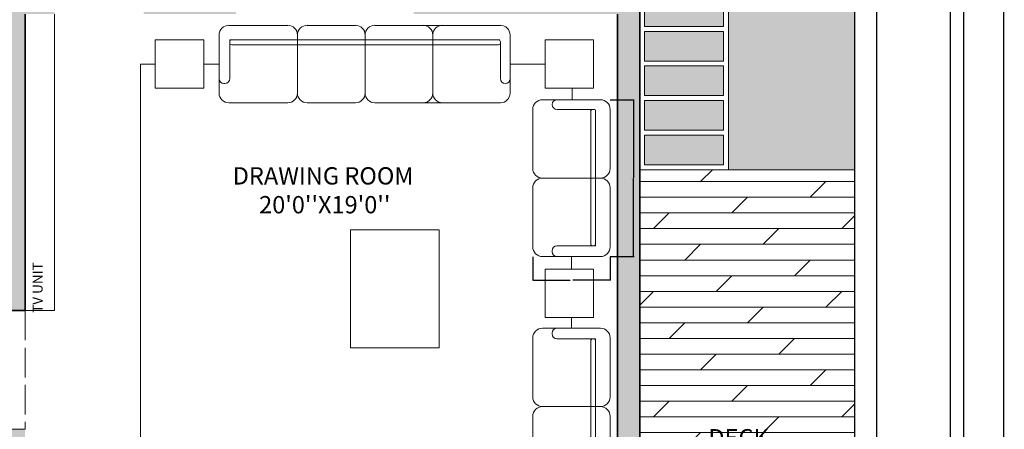
# Model space of a CAD drawing. Units: inches. Extents: x 84 to 1044, y -280 to 906.
# Tile 66 of 105: x 645 to 1044, y 160 to 326. Entities that reach past the tile are written whole.
import ezdxf

# ---------------------------------------------------------------- set-up
doc = ezdxf.new("R2010")
doc.units = ezdxf.units.IN
doc.linetypes.add('ACAD_ISO02W100', pattern=[15, 12, -3])
for name, color, linetype, lineweight in [('A-ANNO-DIMS', 2, 'Continuous', 18), ('A-ANNO-TEXT', 7, 'Continuous', 13), ('A-ANNO-TTLB', 7, 'Continuous', 25), ('A-AREA-IDEN', 7, 'Continuous', 13), ('A-FLOR-CASE', 8, 'Continuous', 18), ('A-FURN', 8, 'Continuous', 15), ('A-WALL-OVHD', 8, 'ACAD_ISO02W100', 13), ('C-PROP', 7, 'Continuous', 25), ('L-HRDS', 32, 'Continuous', 18), ('WALL', 250, 'Continuous', 35)]:
    doc.layers.add(name, color=color, linetype=linetype, lineweight=lineweight)
for name, color, linetype, lineweight, true_color in [('A-FLOR-PATT', 251, 'Continuous', 9, 0x705861), ('A-WALL-PATT', 251, 'Continuous', 9, 0x636466), ('L-HRDS-PATT', 23, 'Continuous', 9, 0xc2877b), ('L-PLNT-PATT', 9, 'Continuous', 9, 0xafd9aa)]:
    doc.layers.add(name, color=color, linetype=linetype, lineweight=lineweight, true_color=true_color)
doc.styles.add('1-100DIM', font='txt', dxfattribs={"height": 0.3})
doc.styles.get("Standard").update_dxf_attribs({"font": 'arial.ttf'})
doc.dimstyles.get("Standard").update_dxf_attribs({"dimtxt": 0.18, "dimasz": 0.18, "dimexe": 0.18, "dimexo": 0.0625, "dimgap": 0.09, "dimtad": 0, "dimtih": 1, "dimtoh": 1, "dimdec": 4, "dimzin": 0, "dimdsep": 46, "dimtxsty": 'Standard', "dimcen": 0.09, "dimadec": 0, "dimazin": 0, "dimtfac": 1, "dimtdec": 4, "dimtofl": 0, "dimtmove": 0, "dimatfit": 3, "dimfxl": 1, "dimtolj": 1, "dimtzin": 0, "dimarcsym": 0})

# ---------------------------------------------------------------- blocks, each defined once
blk = doc.blocks.new('SOFA-4-SEAT')
for p, q in [((3.92, 31.33), (27.81, 31.33)), ((27.81, 31.33), (27.81, 31.33)), ((35.65, 31.33), (55.23, 31.33)), ((55.23, 31.33), (55.23, 31.33)), ((63.07, 31.33), (113.96, 31.33)), ((113.96, 31.33), (113.96, 31.33)), ((0, 3.91), (0, 27.42)), ((4.31, 12.82), (4.31, 25.46)), ((4.31, 25.46), (11.69, 25.46)), ((4.31, 24.28), (4.31, 24.67)), ((5.09, 25.46), (11.69, 25.46)), ((11.69, 25.46), (113.76, 25.46)), ((11.69, 25.46), (113.18, 25.46)), ((31.73, 27.42), (31.73, 3.91)), ((31.73, 3.91), (31.73, 27.42)), ((59.15, 3.91), (59.15, 27.42)), ((59.15, 27.42), (59.15, 3.91)), ((86.57, 27.42), (86.57, 3.91)), ((113.96, 24.67), (113.96, 24.28)), ((113.96, 24.28), (113.96, 9.79)), ((117.88, 27.42), (117.88, 3.91)), ((13.66, 23.5), (5.09, 23.5)), ((113.18, 23.5), (13.66, 23.5)), ((4.31, 9.79), (4.31, 12.82)), ((1.96, 7.83), (2.35, 7.83)), ((115.92, 7.83), (115.92, 7.83)), ((27.81, 0), (3.92, 0)), ((27.81, 0), (27.81, 0)), ((55.23, 0), (35.65, 0)), ((55.23, 0), (55.23, 0)), ((113.96, 0), (63.07, 0)), ((113.96, 0), (113.96, 0))]:
    blk.add_line(p, q)
for centre, radius, start, end in [((3.92, 27.42), 3.92, 90, 180), ((27.81, 27.42), 3.92, 0, 90), ((35.65, 27.42), 3.92, 90, 180), ((55.23, 27.42), 3.92, 0, 90), ((63.07, 27.42), 3.92, 90, 180), ((82.65, 27.42), 3.92, 0, 90), ((90.48, 27.42), 3.92, 90, 180), ((113.96, 27.42), 3.92, 0, 90), ((5.09, 24.67), 0.783, 90, 180), ((5.09, 24.28), 0.783, 180, 270), ((113.18, 24.67), 0.783, 0, 90), ((113.18, 24.28), 0.783, 270, 0), ((1.96, 9.79), 1.96, 180, 270), ((2.35, 9.79), 1.96, 270, 0), ((115.92, 9.79), 1.96, 180, 270), ((115.92, 9.79), 1.96, 270, 0), ((3.92, 3.91), 3.92, 180, 270), ((27.81, 3.91), 3.92, 270, 0), ((35.65, 3.91), 3.92, 180, 270), ((55.23, 3.91), 3.92, 270, 0), ((63.07, 3.91), 3.92, 180, 270), ((82.65, 3.91), 3.92, 270, 0), ((90.48, 3.91), 3.92, 180, 270), ((113.96, 3.91), 3.92, 270, 0)]:
    blk.add_arc(centre, radius, start, end)
blk = doc.blocks.new('SOFA-2-SEAT')
for p, q in [((27.42, 63.46), (3.92, 63.46)), ((7.83, 61.5), (7.83, 61.5)), ((0, 59.54), (0, 59.54)), ((0, 59.54), (0, 35.65)), ((24.29, 59.54), (9.79, 59.54)), ((23.5, 58.76), (23.5, 13.66)), ((24.68, 59.54), (24.29, 59.54)), ((25.46, 11.69), (25.46, 59.35)), ((25.46, 11.69), (25.46, 58.76)), ((31.34, 59.54), (31.34, 59.54)), ((31.34, 35.65), (31.34, 59.54)), ((3.92, 31.73), (27.42, 31.73)), ((27.42, 31.73), (3.92, 31.73)), ((0, 27.81), (0, 27.81)), ((0, 27.81), (0, 3.92)), ((31.34, 27.81), (31.34, 27.81)), ((31.34, 3.92), (31.34, 27.81)), ((23.5, 13.66), (23.5, 5.09)), ((25.46, 5.09), (25.46, 11.69)), ((25.46, 4.31), (25.46, 11.69)), ((9.79, 4.31), (12.83, 4.31)), ((12.83, 4.31), (25.46, 4.31)), ((24.29, 4.31), (24.68, 4.31)), ((3.92, 0), (27.42, 0)), ((7.83, 1.96), (7.83, 2.35))]:
    blk.add_line(p, q)
for centre, radius, start, end in [((3.92, 59.54), 3.92, 90, 180), ((9.79, 61.5), 1.96, 90, 180), ((9.79, 61.5), 1.96, 180, 270), ((27.42, 59.54), 3.92, 360, 90), ((24.29, 58.76), 0.783, 90, 180), ((24.68, 58.76), 0.783, 360, 90), ((3.92, 35.65), 3.92, 180, 270), ((27.42, 35.65), 3.92, 270, 360), ((3.92, 27.81), 3.92, 90, 180), ((27.42, 27.81), 3.92, 360, 90), ((9.79, 2.35), 1.96, 90, 180), ((24.29, 5.09), 0.783, 180, 270), ((24.68, 5.09), 0.783, 270, 360), ((3.92, 3.92), 3.92, 180, 270), ((9.79, 1.96), 1.96, 180, 270), ((27.42, 3.92), 3.92, 270, 360)]:
    blk.add_arc(centre, radius, start, end)
blk = doc.blocks.new('TABLE-END-SQUARE')
for p, q in [((0, 0), (0, 19.59)), ((0, 19.59), (19.58, 19.59)), ((19.58, 19.59), (19.58, 0)), ((19.58, 0), (0, 0))]:
    blk.add_line(p, q)
blk = doc.blocks.new('PAVER-32X12')
blk.add_lwpolyline([(0, 12), (32, 12), (32, 0), (0, 0)], close=True)
blk = doc.blocks.new('*D54')
at = {"layer": 'A-ANNO-DIMS', "color": 0, "lineweight": -2, "transparency": 16777216}
for p, q in [((884.17, 293.48), (893.8, 293.48)), ((893.62, 293.3), (893.62, 261.93)), ((893.62, 230.2), (893.62, 261.57)), ((884.17, 230.02), (893.8, 230.02))]:
    blk.add_line(p, q, dxfattribs=at)
at = {"layer": 'A-ANNO-DIMS', "color": 0, "transparency": 16777216}
for points in [[(893.59, 293.3), (893.65, 293.3), (893.62, 293.48)], [(893.59, 230.2), (893.65, 230.2), (893.62, 230.02)]]:
    blk.add_solid(points, dxfattribs=at)
at = {"layer": 'Defpoints', "color": 0, "transparency": 16777216}
for p in [(884.11, 293.48), (893.62, 293.48), (884.11, 230.02)]:
    blk.add_point(p, dxfattribs=at)
at = {"layer": 'A-ANNO-DIMS', "color": 0, "transparency": 16777216, "insert": (893.62, 261.75), "char_height": 0.18, "attachment_point": 5}
blk.add_mtext('\\A1;LOVESEAT 63 TYP.', dxfattribs=at)
blk = doc.blocks.new('*D55')
at = {"layer": 'A-ANNO-DIMS', "color": 0, "lineweight": -2, "transparency": 16777216}
for p, q in [((852.77, 229.96), (852.77, 220.32)), ((884.11, 229.96), (884.11, 220.32)), ((852.95, 220.5), (867.91, 220.5)), ((883.93, 220.5), (868.97, 220.5))]:
    blk.add_line(p, q, dxfattribs=at)
at = {"layer": 'A-ANNO-DIMS', "color": 0, "transparency": 16777216}
for points in [[(852.95, 220.53), (852.95, 220.47), (852.77, 220.5)], [(883.93, 220.53), (883.93, 220.47), (884.11, 220.5)]]:
    blk.add_solid(points, dxfattribs=at)
at = {"layer": 'Defpoints', "color": 0, "transparency": 16777216}
for p in [(852.77, 230.02), (884.11, 230.02), (884.11, 220.5)]:
    blk.add_point(p, dxfattribs=at)
at = {"layer": 'A-ANNO-DIMS', "color": 0, "transparency": 16777216, "insert": (868.44, 220.5), "char_height": 0.18, "attachment_point": 5}
blk.add_mtext('\\A1;31 TYP.', dxfattribs=at)
blk = doc.blocks.new('*D63')
at = {"layer": 'A-ANNO-DIMS', "color": 0, "lineweight": -2, "transparency": 16777216}
for p, q in [((833.14, 709.12), (1043.77, 709.12)), ((1043.59, 708.94), (1043.59, 400.3)), ((1043.59, 91.3), (1043.59, 399.94)), ((896.14, 91.12), (1043.77, 91.12))]:
    blk.add_line(p, q, dxfattribs=at)
at = {"layer": 'A-ANNO-DIMS', "color": 0, "transparency": 16777216}
for points in [[(1043.56, 708.94), (1043.62, 708.94), (1043.59, 709.12)], [(1043.56, 91.3), (1043.62, 91.3), (1043.59, 91.12)]]:
    blk.add_solid(points, dxfattribs=at)
at = {"layer": 'Defpoints', "color": 0, "transparency": 16777216}
for p in [(833.07, 709.12), (1043.59, 709.12), (896.07, 91.12)]:
    blk.add_point(p, dxfattribs=at)
at = {"layer": 'A-ANNO-DIMS', "color": 0, "transparency": 16777216, "insert": (1043.59, 400.12), "char_height": 0.18, "attachment_point": 5}
blk.add_mtext('\\A1;618', dxfattribs=at)

msp = doc.modelspace()

# ---------------------------------------------------------------- hatches: boundary and pattern name
at = {"layer": 'A-FLOR-PATT', "transparency": 33554597}
h = msp.add_hatch(dxfattribs=at)
h.set_pattern_fill('DOLMIT', color=256)
h.paths.add_polyline_path([(983.074, 265.12), (896.074, 265.12), (896.074, 91.12), (887.074, 91.12), (887.074, 31.12), (983.074, 31.12)])
at = {"layer": 'A-WALL-PATT', "transparency": 33554597}
h = msp.add_hatch(color=256, dxfattribs=at)
h.dxf.hatch_style = 1
h.paths.add_polyline_path([(671.074, 100.12), (647.074, 100.12), (647.074, 160.12), (641.074, 160.12), (620.824, 160.12), (620.824, 151.12), (638.074, 151.12), (638.074, 91.12), (671.074, 91.12)])
h.paths.add_polyline_path([(791.074, 100.12), (743.074, 100.12), (743.074, 91.12), (791.074, 91.12)])
h.paths.add_polyline_path([(896.074, 346.12), (887.074, 346.12), (887.074, 334.12), (870.955, 334.12), (833.074, 334.12), (804.574, 334.12), (804.574, 328.12), (887.074, 328.12), (887.074, 100.12), (863.074, 100.12), (863.074, 91.12), (896.074, 91.12)])
h.paths.add_polyline_path([(507.574, 154.729), (507.574, 160.12), (464.074, 160.12), (464.074, 247.12), (641.074, 247.12), (641.074, 208.12), (647.074, 208.12), (647.074, 328.12), (659.074, 328.12), (659.074, 334.12), (617.074, 334.12), (617.074, 328.12), (641.074, 328.12), (641.074, 256.12), (545.074, 256.12), (545.074, 328.12), (569.074, 328.12), (569.074, 334.12), (518.074, 334.12), (518.074, 325.12), (536.074, 325.12), (536.074, 256.12), (464.074, 256.12), (464.074, 325.12), (482.074, 325.12), (482.074, 334.12), (455.074, 334.12), (455.074, 160.12), (413.127, 160.12), (413.127, 151.12), (455.074, 151.12), (455.074, 91.12), (464.074, 91.12), (464.074, 151.12), (507.574, 151.12)])
h.paths.add_polyline_path([(572.824, 160.12), (555.574, 160.12), (555.574, 151.12), (572.824, 151.12)], flags=17)
h.paths.add_polyline_path([(341.127, 160.12), (299.179, 160.12), (299.179, 211.12), (294.179, 211.12), (290.179, 211.12), (290.179, 151.12), (341.127, 151.12)])
h.paths.add_polyline_path([(299.179, 256.12), (212.179, 256.12), (212.179, 274.12), (203.179, 274.12), (203.179, 247.12), (299.179, 247.12)])
h.paths.add_polyline_path([(212.179, 514.12), (398.074, 514.12), (398.074, 519.12), (398.074, 520.12), (212.179, 520.12), (212.179, 574.12), (203.179, 574.12), (203.179, 310.12), (212.179, 310.12), (212.179, 328.12), (290.179, 328.12), (290.179, 292.12), (299.179, 292.12), (299.179, 328.12), (332.179, 328.12), (332.179, 334.12), (212.179, 334.12)])
h.paths.add_polyline_path([(287.127, 709.12), (203.179, 709.12), (203.179, 646.12), (212.179, 646.12), (212.179, 700.12), (287.127, 700.12)])
h.paths.add_polyline_path([(470.074, 709.12), (359.127, 709.12), (359.127, 700.12), (434.074, 700.12), (434.074, 574.12), (440.074, 574.12), (440.074, 622.12), (464.074, 622.12), (464.074, 628.12), (440.074, 628.12), (440.074, 700.12), (470.074, 700.12)])
h.paths.add_polyline_path([(572.074, 709.12), (506.074, 709.12), (506.074, 700.12), (536.074, 700.12), (536.074, 628.12), (494.074, 628.12), (494.074, 622.12), (536.074, 622.12), (536.074, 520.12), (440.074, 520.12), (440.074, 544.12), (434.074, 544.12), (434.074, 514.12), (644.074, 514.12), (644.074, 519.12), (644.074, 544.12), (638.074, 544.12), (638.074, 520.12), (542.074, 520.12), (542.074, 622.12), (584.074, 622.12), (584.074, 628.12), (542.074, 628.12), (542.074, 700.12), (572.074, 700.12)])
h.paths.add_polyline_path([(698.074, 709.12), (608.074, 709.12), (608.074, 700.12), (638.074, 700.12), (638.074, 628.12), (614.074, 628.12), (614.074, 622.12), (638.074, 622.12), (638.074, 574.12), (644.074, 574.12), (644.074, 700.12), (698.074, 700.12)])
h.paths.add_polyline_path([(833.074, 709.12), (770.074, 709.12), (770.074, 700.12), (824.074, 700.12), (824.074, 646.12), (833.074, 646.12)])
h.paths.add_polyline_path([(833.074, 574.12), (824.074, 574.12), (824.074, 520.12), (791.244, 520.12), (712.904, 520.12), (680.074, 520.12), (680.074, 514.12), (695.074, 514.12), (695.074, 491.62), (704.074, 491.62), (704.074, 511.12), (833.074, 511.12)])
h.paths.add_polyline_path([(704.074, 419.62), (695.074, 419.62), (695.074, 370.12), (704.074, 370.12)])
h.paths.add_polyline_path([(896.074, 400.12), (833.074, 400.12), (833.074, 364.12), (839.074, 364.12), (839.074, 394.12), (887.074, 394.12), (887.074, 382.12), (896.074, 382.12)])
h.paths.add_polyline_path([(732.574, 334.12), (695.074, 334.12), (695.074, 328.12), (732.574, 328.12)])
at = {"layer": 'L-HRDS-PATT', "transparency": 33554597}
h = msp.add_hatch(color=256, dxfattribs=at)
h.dxf.hatch_style = 1
h.paths.add_polyline_path([(930.074, 545.12), (898.074, 545.12), (898.074, 533.12), (930.074, 533.12)])
h.paths.add_polyline_path([(930.074, 531.12), (898.074, 531.12), (898.074, 519.12), (930.074, 519.12)])
h.paths.add_polyline_path([(930.074, 517.12), (898.074, 517.12), (898.074, 505.12), (930.074, 505.12)])
h.paths.add_polyline_path([(930.074, 503.12), (898.074, 503.12), (898.074, 491.12), (930.074, 491.12)])
h.paths.add_polyline_path([(930.074, 489.12), (898.074, 489.12), (898.074, 477.12), (930.074, 477.12)])
h.paths.add_polyline_path([(930.074, 475.12), (898.074, 475.12), (898.074, 463.12), (930.074, 463.12)])
h.paths.add_polyline_path([(930.074, 461.12), (898.074, 461.12), (898.074, 449.12), (930.074, 449.12)])
h.paths.add_polyline_path([(930.074, 447.12), (898.074, 447.12), (898.074, 435.12), (930.074, 435.12)])
h.paths.add_polyline_path([(930.074, 433.12), (898.074, 433.12), (898.074, 421.12), (930.074, 421.12)])
h.paths.add_polyline_path([(930.074, 419.12), (898.074, 419.12), (898.074, 407.12), (930.074, 407.12)])
h.paths.add_polyline_path([(930.074, 405.12), (898.074, 405.12), (898.074, 393.12), (930.074, 393.12)])
h.paths.add_polyline_path([(930.074, 391.12), (898.074, 391.12), (898.074, 379.12), (930.074, 379.12)])
h.paths.add_polyline_path([(930.074, 377.12), (898.074, 377.12), (898.074, 365.12), (930.074, 365.12)])
h.paths.add_polyline_path([(930.074, 363.12), (898.074, 363.12), (898.074, 351.12), (930.074, 351.12)])
h.paths.add_polyline_path([(930.074, 349.12), (898.074, 349.12), (898.074, 337.12), (930.074, 337.12)])
h.paths.add_polyline_path([(930.074, 335.12), (898.074, 335.12), (898.074, 323.12), (930.074, 323.12)])
h.paths.add_polyline_path([(930.074, 321.12), (898.074, 321.12), (898.074, 309.12), (930.074, 309.12)])
h.paths.add_polyline_path([(930.074, 307.12), (898.074, 307.12), (898.074, 295.12), (930.074, 295.12)])
h.paths.add_polyline_path([(930.074, 293.12), (898.074, 293.12), (898.074, 281.12), (930.074, 281.12)])
h.paths.add_polyline_path([(930.074, 279.12), (898.074, 279.12), (898.074, 267.12), (930.074, 267.12)])
at = {"layer": 'L-PLNT-PATT', "transparency": 33554597}
h = msp.add_hatch(color=256, dxfattribs=at)
h.dxf.hatch_style = 1
h.paths.add_polyline_path([(434.074, 769.12), (386.074, 769.12), (386.074, 709.12), (434.074, 709.12)])
h.paths.add_polyline_path([(896.074, 847.12), (434.074, 847.12), (434.074, 769.12), (434.074, 709.12), (470.074, 709.12), (506.074, 709.12), (572.074, 709.12), (608.074, 709.12), (698.074, 709.12), (770.074, 709.12), (833.074, 709.12), (896.074, 709.12)])
h.paths.add_polyline_path([(983.074, 847.12), (896.074, 847.12), (896.074, 709.12), (896.074, 547.12), (932.074, 547.12), (983.074, 547.12)])
h.paths.add_polyline_path([(983.074, 547.12), (932.074, 547.12), (932.074, 265.12), (983.074, 265.12)])
h.paths.add_polyline_path([(203.179, 646.12), (203.179, 709.12), (203.179, 745.12), (143.179, 745.12), (143.179, 271.12), (203.179, 271.12), (203.179, 274.12), (203.179, 310.12), (203.179, 574.12)])

# ---------------------------------------------------------------- linework, layer by layer
at = {"layer": 'A-ANNO-TTLB'}
for points in [[(101.1, 905.916), (1027.308, 905.916), (1027.308, -279.764), (101.1, -279.764)], [(106.576, 900.439), (1021.832, 900.439), (1021.832, -274.288), (106.576, -274.288)]]:
    msp.add_lwpolyline(points, close=True, dxfattribs=at)
at = {"layer": 'A-FLOR-CASE'}
for p in [(659.074, 328.12), (647.074, 208.12)]:
    msp.add_line(p, (659.074, 208.12), dxfattribs=at)
at = {"layer": 'A-FURN'}
for p, q in [((699.863, 307.895), (693.863, 307.895)), ((693.863, 307.895), (693.863, 122.358)), ((719.448, 307.895), (725.702, 307.895)), ((843.576, 307.895), (857.76, 307.895)), ((868.727, 298.103), (868.727, 293.478)), ((778.938, 193.133), (778.938, 240.835)), ((778.938, 240.835), (814.829, 240.835)), ((814.829, 240.835), (814.829, 193.133)), ((868.438, 230.023), (868.438, 224.921)), ((868.438, 205.336), (868.438, 201.023)), ((814.829, 193.133), (778.938, 193.133))]:
    msp.add_line(p, q, dxfattribs=at)
at = {"layer": 'A-WALL-OVHD'}
msp.add_lwpolyline([(641.074, 208.12), (647.074, 208.12), (647.074, 160.12), (641.074, 160.12)], close=True, dxfattribs=at)
at = {"layer": 'C-PROP'}
for points in [[(143.179, -121.88), (134.179, -121.88), (134.179, 856.12), (992.074, 856.12), (992.074, -121.88), (624.574, -121.88)], [(143.179, -112.88), (143.179, 847.12), (983.074, 847.12), (983.074, -112.88), (624.574, -112.88)]]:
    msp.add_lwpolyline(points, dxfattribs=at)
at = {"layer": 'L-HRDS'}
for p, q in [((932.074, 265.12), (932.074, 547.12)), ((896.074, 265.12), (983.074, 265.12))]:
    msp.add_line(p, q, dxfattribs=at)
at = {"layer": 'WALL'}
for p, q in [((896.074, 91.12), (896.074, 346.12)), ((647.074, 328.12), (647.074, 208.12)), ((887.074, 100.12), (887.074, 328.12)), ((641.074, 208.12), (647.074, 208.12))]:
    msp.add_line(p, q, dxfattribs=at)

# ---------------------------------------------------------------- block references
at = {"layer": 'A-FURN'}
for name, p in [('SOFA-4-SEAT', (725.7, 292.23)), ('TABLE-END-SQUARE', (857.76, 298.1)), ('SOFA-2-SEAT', (852.77, 230.02)), ('TABLE-END-SQUARE', (857.76, 205.333))]:
    msp.add_blockref(name, p, dxfattribs=at)
at = {"layer": 'A-FURN', "rotation": 90.00000000012837}
msp.add_blockref('TABLE-END-SQUARE', (719.451, 298.103), dxfattribs=at)
at = {"layer": 'A-FURN', "extrusion": (0, 0, -1), "zscale": -1, "rotation": 180}
msp.add_blockref('SOFA-2-SEAT', (-852.77, 201.026), dxfattribs=at)
at = {"layer": 'L-HRDS', "extrusion": (0, 0, -1), "zscale": -1, "rotation": 180}
for p in [(-898.07, 335.12), (-898.07, 321.12), (-898.07, 307.12), (-898.07, 293.12), (-898.07, 279.12)]:
    msp.add_blockref('PAVER-32X12', p, dxfattribs=at)

# ---------------------------------------------------------------- texts
at = {"layer": 'A-ANNO-TEXT', "insert": (650.17, 205.132), "char_height": 7, "attachment_point": 1, "rotation": 90, "style": '1-100DIM'}
msp.add_mtext_dynamic_manual_height_columns('{\\f@Malgun Gothic|b0|i0|c0|p34; \\H0.57143x;TV UNIT}', width=25.324, gutter_width=15.851, heights=[0], dxfattribs=at)
at = {"layer": 'A-AREA-IDEN', "char_height": 7, "attachment_point": 1, "style": '1-100DIM'}
for s, width, insert in [("{\\f@Malgun Gothic|b0|i0|c0|p34;DRAWING ROOM\\P     20'0''X19'0''}", 95.09774, (731.21, 266.161)), ('{\\f@Malgun Gothic|b0|i0|c0|p34;    DECK }', 51.07953, (915.356, 160.191))]:
    msp.add_mtext_dynamic_manual_height_columns(s, width=width, gutter_width=15.851, heights=[0], dxfattribs=dict(at, insert=insert))

# ---------------------------------------------------------------- dimensions: what is measured, and where the dimension line sits
at = {"layer": 'A-ANNO-DIMS'}
dim = msp.add_linear_dim(base=(1043.588, 709.12), p1=(896.074, 91.12), p2=(833.074, 709.12), angle=90, dimstyle='Standard', override={"dimdec": 0, "dimlfac": 1, "dimrnd": 0, "dimzin": 0, "dimdsep": 46, "dimlunit": 2}, dxfattribs=at)
dim.commit()
dim.dimension.update_dxf_attribs({"geometry": '*D63', "text_midpoint": (1043.588, 400.12)})
dim = msp.add_linear_dim(base=(893.625, 293.478), p1=(884.106, 230.023), p2=(884.106, 293.478), angle=90, text='LOVESEAT <> TYP.', dimstyle='Standard', override={"dimdec": 0, "dimlfac": 1, "dimrnd": 0, "dimzin": 0, "dimdsep": 46, "dimlunit": 2}, dxfattribs=at)
dim.commit()
dim.dimension.update_dxf_attribs({"geometry": '*D54', "text_midpoint": (893.625, 261.751)})
dim = msp.add_linear_dim(base=(884.106, 220.505), p1=(852.77, 230.023), p2=(884.106, 230.023), text='<> TYP.', dimstyle='Standard', override={"dimdec": 0, "dimlfac": 1, "dimrnd": 0, "dimzin": 0, "dimdsep": 46, "dimlunit": 2}, dxfattribs=at)
dim.commit()
dim.dimension.update_dxf_attribs({"geometry": '*D55', "text_midpoint": (868.438, 220.505)})

doc.saveas('drawing.dxf')
